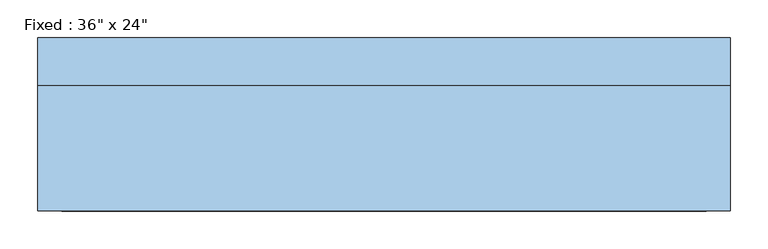
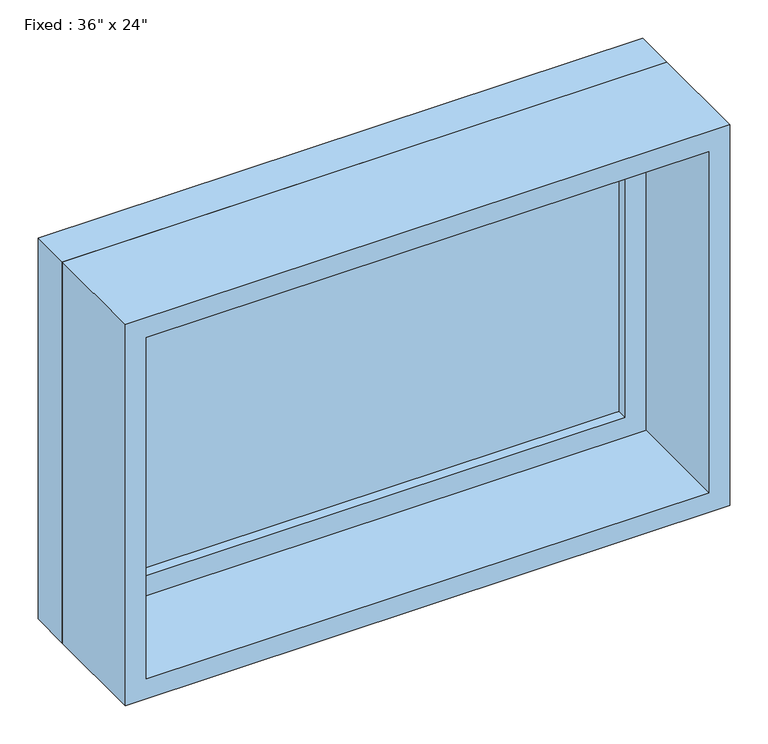
"""IFC4 building model written with IfcOpenShell, lengths in millimetres: window geometry."""

from ifc_helpers import new_model, si_unit, frame, origin, place, context, project, spatial, polyline, outline, extrude, source, transform, mapped, element, save


def window_bb95b1c9(model_context):
    return source(origin(), model_context, "Body", "SweptSolid", [
        extrude(outline(polyline([(355.6, 66.675), (-431.8, 66.675), (-431.8, 79.375), (355.6, 79.375), (355.6, 66.675)])), frame((0.0, 0.0, 977.9), z_axis=(0.0, 0.0, 1.0), x_axis=(1.0, 0.0, 0.0)), (0.0, 0.0, 1.0), 482.6),
        extrude(outline(polyline([(1504.95, -476.25), (933.45, -476.25), (933.45, 400.05), (1504.95, 400.05), (1504.95, -476.25)]), holes=[polyline([(1460.5, -431.8), (1460.5, 355.6), (977.9, 355.6), (977.9, -431.8), (1460.5, -431.8)])]), frame((0.0, 50.8, 0.0), z_axis=(0.0, 1.0, 0.0), x_axis=(0.0, 0.0, 1.0)), (0.0, 0.0, 1.0), 44.45),
        extrude(outline(polyline([(1524.0, -495.3), (914.4, -495.3), (914.4, 419.1), (1524.0, 419.1), (1524.0, -495.3)]), holes=[polyline([(1492.25, -463.55), (1492.25, 387.35), (946.15, 387.35), (946.15, -463.55), (1492.25, -463.55)])]), frame((0.0, -114.3, 0.0), z_axis=(0.0, 1.0, 0.0), x_axis=(0.0, 0.0, 1.0)), (0.0, 0.0, 1.0), 165.1),
        extrude(outline(polyline([(1524.0, 419.1), (1524.0, -495.3), (914.4, -495.3), (914.4, 419.1), (1524.0, 419.1)]), holes=[polyline([(1504.95, 400.05), (933.45, 400.05), (933.45, -476.25), (1504.95, -476.25), (1504.95, 400.05)])]), frame((0.0, 50.8, 0.0), z_axis=(0.0, 1.0, 0.0), x_axis=(0.0, 0.0, 1.0)), (0.0, 0.0, 1.0), 63.5),
    ])


if __name__ == "__main__":
    model = new_model("IFC4")
    model_context = context("Model", 3, world=origin())
    ifc_project = project(units=[si_unit("LENGTHUNIT", "METRE", prefix="MILLI")], contexts=[model_context])
    site = spatial("IfcSite", under=ifc_project)
    building = spatial("IfcBuilding", under=site)
    placement = place(None, origin())
    window_shape = window_bb95b1c9(model_context)
    element("IfcWindow", 1, ObjectType="Fixed : 36\" x 24\"", at=placement, inside=building, context=model_context, shape_type="MappedRepresentation", body=[
        mapped(window_shape, transform((0.0, 0.0, 0.0), x_axis=(1.0, 0.0, 0.0), y_axis=(0.0, 1.0, 0.0), z_axis=(0.0, 0.0, 1.0))),
    ])
    save(model, "model.ifc")

# Revit data of these elements
# Type "Fixed : 36\" x 24\""
#   Type Mark = "8"
#   Construction Type Id = "GSP4R"
#   Assembly Code = "B2020100"
#   Analytic Construction = "1/8 in Pilkington single glazing"
#   Visual Light Transmittance = 0.9
#   Solar Heat Gain Coefficient = 0.78
#   Heat Transfer Coefficient (U) = 0.6496 BTU/(h·ft²·°F)
#   Height = 2' - 0"
#   Default Sill Height = 3' - 0"
#   Width = 3' - 0"
#   Window Inset = 0' - 0 3/4"
#   Define Thermal Properties by = 1
#   Define Thermal Properties by = 1
#   Glass Pane Material = Glass
#   Sash Material = Sash
#   Wall Closure = (empty or 0)
# Element 1 (IfcWindow, "Fixed : 36\" x 24\"")
#   Materials on its faces: "Sash", "Glass"
# Materials
#   "Glass": class "Glass", colour RGB 0 128 192, transparency 0.75, Description = "Soda Lime Glass", Cost = 0
#   "Sash": class "Wood", colour RGB 224 178 126, transparency 0, Cost = 0
